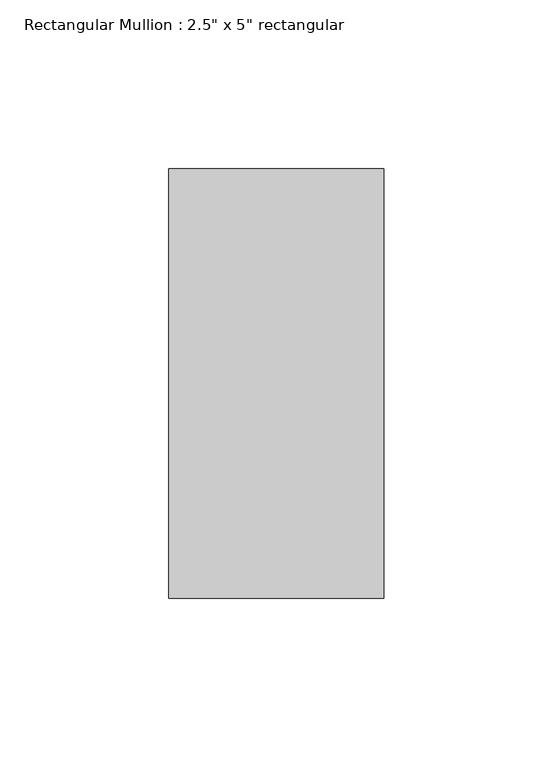
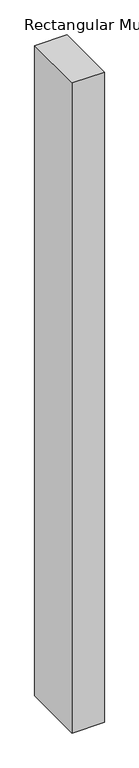
"""IFC4 building model written with IfcOpenShell, lengths in millimetres: member geometry."""

from ifc_helpers import new_model, si_unit, frame, origin, place, context, project, spatial, polyline, outline, extrude, source, transform, mapped, element, save


def member_cd571718(model_context):
    return source(origin(), model_context, "Body", "SweptSolid", [
        extrude(outline(polyline([(0.0, 63.5), (0.0, -63.5), (-63.5, -63.5), (-63.5, 63.5), (0.0, 63.5)])), frame((0.0, 0.0, -1350.2562894), z_axis=(0.0, 0.0, 1.0), x_axis=(1.0, 0.0, 0.0)), (0.0, 0.0, 1.0), 1350.2562894),
    ])


if __name__ == "__main__":
    model = new_model("IFC4")
    model_context = context("Model", 3, world=origin())
    ifc_project = project(units=[si_unit("LENGTHUNIT", "METRE", prefix="MILLI")], contexts=[model_context])
    site = spatial("IfcSite", under=ifc_project)
    building = spatial("IfcBuilding", under=site)
    placement = place(None, origin())
    member_shape = member_cd571718(model_context)
    element("IfcMember", 1, ObjectType="Rectangular Mullion : 2.5\" x 5\" rectangular", at=placement, inside=building, context=model_context, shape_type="MappedRepresentation", body=[
        mapped(member_shape, transform((0.0, 0.0, 0.0), x_axis=(1.0, 0.0, 0.0), y_axis=(0.0, 1.0, 0.0), z_axis=(0.0, 0.0, 1.0))),
    ])
    save(model, "model.ifc")

# Revit data of these elements
# Type "Rectangular Mullion : 2.5\" x 5\" rectangular"
#   built-in parameter 1007304 = 0.416667 (stored number, unit not read)
#   built-in parameter 1007301 = 0.104167 (stored number, unit not read)
#   built-in parameter 1007300 = 0.104167 (stored number, unit not read)
# Element 1 (IfcMember, "Rectangular Mullion : 2.5\" x 5\" rectangular")
#   Materials on its faces: "door colour"
# Materials
#   "door colour": class "Generic", colour RGB 120 120 120, transparency 0, Cost = 0
